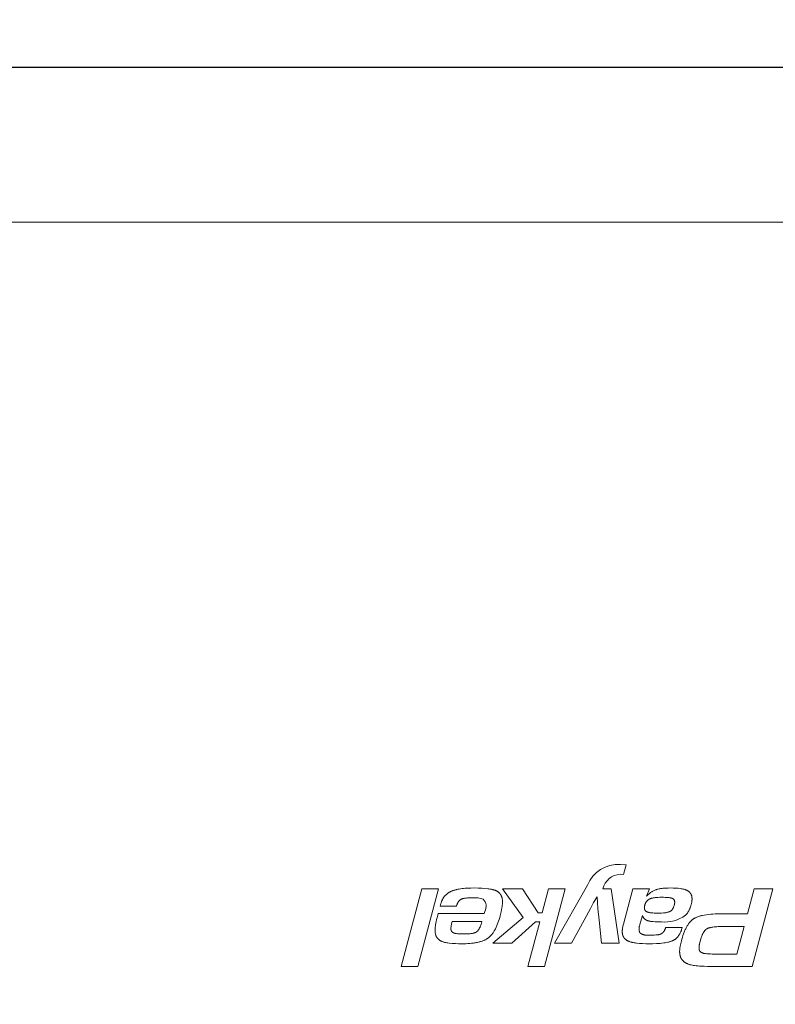
# Model space of a CAD drawing. Units: inches. Extents: x -1198 to -69, y -512 to 437.
# Tile 11 of 50: x -950.733 to -948.245, y 182.142 to 185.385. Entities that reach past the tile are written whole.
import ezdxf

# ---------------------------------------------------------------- set-up
doc = ezdxf.new("R2010")
doc.units = ezdxf.units.IN
doc.header["$MEASUREMENT"] = 0
for name, color, linetype, lineweight in [('0_Pen_No__7', 7, 'Continuous', 18), ('A-ANNO-DIMS', 2, 'Continuous', 18), ('A-EQPM', 60, 'Continuous', 18), ('A-FLOR-CASE', 7, 'Continuous', 25)]:
    doc.layers.add(name, color=color, linetype=linetype, lineweight=lineweight)
doc.styles.get("Standard").update_dxf_attribs({"font": 'arial.ttf'})
doc.dimstyles.get("Standard").update_dxf_attribs({"dimtxt": 6, "dimasz": 6, "dimexe": 0.18, "dimexo": 0.0625, "dimgap": 0.09, "dimtad": 0, "dimtih": 1, "dimtoh": 1, "dimdec": 0, "dimzin": 0, "dimdsep": 46, "dimlunit": 4, "dimtxsty": 'Standard', "dimblk": 'OBLIQUE', "dimcen": 0.09, "dimadec": 0, "dimazin": 0, "dimtfac": 1, "dimtdec": 0, "dimtofl": 0, "dimtmove": 0, "dimatfit": 3, "dimfxl": 1, "dimtolj": 1, "dimtzin": 0, "dimarcsym": 0})

# ---------------------------------------------------------------- blocks, each defined once
blk = doc.blocks.new('new block')
at = {"layer": '0_Pen_No__7'}
for p, q in [((-281.076, 68.7), (-279.346, 75.2)), ((-279.346, 75.2), (-275.605, 75.2)), ((-263.696, 68.7), (-261.965, 75.2)), ((-261.965, 75.2), (-260.589, 75.2)), ((-260.589, 75.2), (-261.574, 71.478)), ((-253.094, 68.7), (-251.364, 75.2)), ((-249.986, 75.2), (-251.716, 68.7)), ((-251.364, 75.2), (-249.986, 75.2)), ((-278.066, 74.168), (-278.675, 71.867)), ((-276.153, 74.168), (-278.066, 74.168)), ((-267.552, 68.7), (-268.209, 73.251)), ((-268.209, 73.251), (-266.747, 73.251)), ((-266.747, 73.251), (-266.552, 71.321)), ((-262.799, 73.251), (-265.577, 68.417)), ((-265.297, 71.321), (-264.224, 73.251)), ((-264.224, 73.251), (-262.799, 73.251)), ((-261.221, 71.478), (-259.224, 73.251)), ((-257.639, 73.251), (-260.186, 71.107)), ((-259.224, 73.251), (-257.639, 73.251)), ((-278.675, 71.867), (-276.921, 71.867)), ((-272.109, 71.935), (-273.497, 71.935)), ((-270.171, 70.951), (-269.953, 71.692)), ((-268.575, 71.673), (-269.367, 68.7)), ((-254.202, 71.634), (-254.141, 72.033)), ((-266.552, 71.321), (-266.443, 70.356)), ((-265.821, 70.356), (-265.297, 71.321)), ((-261.574, 71.478), (-261.221, 71.478)), ((-260.186, 71.107), (-258.444, 68.7)), ((-256.736, 71.458), (-254.251, 71.458)), ((-254.251, 71.458), (-254.202, 71.634)), ((-252.985, 71.146), (-253.081, 70.776)), ((-278.956, 70.795), (-279.517, 68.7)), ((-277.141, 70.795), (-278.956, 70.795)), ((-276.786, 70.805), (-277.141, 70.795)), ((-266.443, 70.356), (-266.393, 69.87)), ((-266.076, 69.87), (-265.821, 70.356)), ((-261.783, 70.717), (-262.318, 68.7)), ((-261.453, 70.717), (-261.783, 70.717)), ((-260.138, 68.7), (-261.453, 70.717)), ((-256.931, 70.776), (-256.98, 70.601)), ((-253.081, 70.776), (-256.931, 70.776)), ((-254.605, 70.152), (-253.239, 70.152)), ((-253.264, 70.065), (-253.277, 70.016)), ((-253.239, 70.152), (-253.264, 70.065)), ((-270.744, 68.7), (-270.512, 69.324)), ((-266.393, 69.87), (-266.37, 69.393)), ((-266.37, 69.393), (-266.076, 69.87)), ((-279.517, 68.7), (-281.076, 68.7)), ((-269.367, 68.7), (-270.744, 68.7)), ((-266.857, 68.7), (-267.552, 68.7)), ((-262.318, 68.7), (-263.696, 68.7)), ((-258.444, 68.7), (-260.138, 68.7)), ((-251.716, 68.7), (-253.094, 68.7)), ((-268.794, 66.703), (-268.575, 67.501)), ((-268.575, 67.501), (-268.307, 67.492)), ((-268.318, 66.683), (-268.794, 66.703))]:
    blk.add_line(p, q, dxfattribs=at)
blk.add_lwpolyline([(-354.492, 596.906), (481.176, 596.906, -0.414214), (485.681, 592.401), (485.681, 99.109), (486.244, 99.109), (486.244, 95.73), (485.681, 95.73), (485.681, 4.505, -0.414214), (481.176, 0), (-354.492, 0, -0.414214), (-358.997, 4.505), (-358.997, 95.73), (-359.56, 95.73), (-359.56, 99.109), (-358.997, 99.109), (-358.997, 592.401, -0.414214)], format="xyb", close=True, dxfattribs=at)
blk.add_lwpolyline([(-333.701, 12.952), (460.296, 12.952), (460.296, 570.439), (-333.701, 570.439)], close=True, dxfattribs=at)
for points in [[(-275.605, 75.2), (-275.335, 75.196), (-275.064, 75.185), (-274.929, 75.176), (-274.794, 75.164), (-274.659, 75.149), (-274.524, 75.132), (-274.432, 75.118), (-274.34, 75.102), (-274.249, 75.084), (-274.204, 75.074), (-274.159, 75.062), (-274.115, 75.05), (-274.071, 75.036), (-274.027, 75.022), (-273.983, 75.006), (-273.94, 74.989), (-273.898, 74.97), (-273.877, 74.96), (-273.856, 74.95), (-273.836, 74.939), (-273.815, 74.928), (-273.785, 74.911), (-273.755, 74.893), (-273.725, 74.874), (-273.696, 74.854), (-273.668, 74.833), (-273.64, 74.811), (-273.613, 74.789), (-273.586, 74.765), (-273.561, 74.741), (-273.537, 74.716), (-273.525, 74.703), (-273.513, 74.69), (-273.502, 74.677), (-273.49, 74.664), (-273.48, 74.65), (-273.469, 74.637), (-273.459, 74.623), (-273.449, 74.609), (-273.439, 74.594), (-273.43, 74.58), (-273.421, 74.565), (-273.412, 74.55), (-273.403, 74.534), (-273.394, 74.517), (-273.385, 74.5), (-273.377, 74.483), (-273.37, 74.466), (-273.362, 74.449), (-273.355, 74.431), (-273.349, 74.414), (-273.342, 74.396), (-273.336, 74.378), (-273.331, 74.36), (-273.326, 74.342), (-273.316, 74.305), (-273.307, 74.268), (-273.3, 74.23), (-273.294, 74.192), (-273.289, 74.154), (-273.285, 74.116), (-273.282, 74.077), (-273.279, 74.039), (-273.278, 74), (-273.277, 73.962), (-273.278, 73.905), (-273.28, 73.848), (-273.283, 73.792), (-273.288, 73.736), (-273.294, 73.68), (-273.302, 73.624), (-273.31, 73.569), (-273.32, 73.513), (-273.342, 73.403), (-273.367, 73.294), (-273.395, 73.185), (-273.425, 73.077)], [(-275.032, 72.969), (-274.96, 73.227), (-274.938, 73.314), (-274.929, 73.357), (-274.92, 73.401), (-274.913, 73.445), (-274.907, 73.489), (-274.902, 73.534), (-274.9, 73.556), (-274.899, 73.579), (-274.898, 73.602), (-274.898, 73.624), (-274.898, 73.647), (-274.898, 73.67), (-274.899, 73.687), (-274.9, 73.704), (-274.901, 73.722), (-274.903, 73.739), (-274.905, 73.756), (-274.908, 73.773), (-274.911, 73.789), (-274.915, 73.806), (-274.919, 73.822), (-274.923, 73.838), (-274.929, 73.854), (-274.935, 73.869), (-274.941, 73.884), (-274.949, 73.899), (-274.957, 73.913), (-274.966, 73.926), (-274.975, 73.938), (-274.984, 73.95), (-274.995, 73.961), (-275.006, 73.972), (-275.017, 73.982), (-275.029, 73.992), (-275.041, 74.002), (-275.054, 74.011), (-275.067, 74.02), (-275.081, 74.028), (-275.094, 74.036), (-275.108, 74.043), (-275.123, 74.05), (-275.137, 74.057), (-275.152, 74.064), (-275.166, 74.07), (-275.189, 74.078), (-275.212, 74.086), (-275.235, 74.094), (-275.258, 74.1), (-275.281, 74.106), (-275.305, 74.112), (-275.328, 74.116), (-275.352, 74.121), (-275.399, 74.128), (-275.446, 74.134), (-275.541, 74.143), (-275.694, 74.154), (-275.847, 74.162), (-276, 74.166), (-276.153, 74.168)], [(-276.921, 71.867), (-276.705, 71.869), (-276.488, 71.876), (-276.38, 71.882), (-276.272, 71.89), (-276.164, 71.901), (-276.056, 71.914), (-275.982, 71.925), (-275.908, 71.938), (-275.871, 71.946), (-275.834, 71.954), (-275.797, 71.963), (-275.761, 71.972), (-275.734, 71.98), (-275.708, 71.988), (-275.682, 71.997), (-275.656, 72.006), (-275.643, 72.011), (-275.63, 72.017), (-275.617, 72.022), (-275.605, 72.028), (-275.593, 72.034), (-275.58, 72.04), (-275.568, 72.047), (-275.556, 72.053), (-275.546, 72.06), (-275.535, 72.067), (-275.524, 72.074), (-275.514, 72.081), (-275.504, 72.089), (-275.494, 72.096), (-275.484, 72.104), (-275.474, 72.112), (-275.464, 72.121), (-275.455, 72.129), (-275.436, 72.146), (-275.418, 72.165), (-275.401, 72.183), (-275.381, 72.206), (-275.362, 72.229), (-275.343, 72.253), (-275.326, 72.277), (-275.309, 72.302), (-275.292, 72.327), (-275.277, 72.353), (-275.261, 72.379), (-275.242, 72.413), (-275.224, 72.449), (-275.206, 72.484), (-275.189, 72.52), (-275.173, 72.556), (-275.157, 72.593), (-275.128, 72.666), (-275.101, 72.741), (-275.077, 72.817), (-275.054, 72.893), (-275.032, 72.969)], [(-273.425, 73.077), (-273.465, 72.926), (-273.508, 72.776), (-273.555, 72.627), (-273.605, 72.479), (-273.66, 72.333), (-273.69, 72.261), (-273.72, 72.189), (-273.752, 72.118), (-273.786, 72.048), (-273.821, 71.978), (-273.857, 71.909), (-273.886, 71.856), (-273.916, 71.805), (-273.948, 71.753), (-273.98, 71.703), (-274.014, 71.653), (-274.049, 71.604), (-274.086, 71.557), (-274.124, 71.51), (-274.157, 71.471), (-274.192, 71.434), (-274.228, 71.397), (-274.264, 71.361), (-274.283, 71.344), (-274.303, 71.327), (-274.322, 71.311), (-274.342, 71.295), (-274.362, 71.279), (-274.382, 71.263), (-274.403, 71.249), (-274.424, 71.234), (-274.446, 71.219), (-274.469, 71.205), (-274.492, 71.191), (-274.515, 71.177), (-274.538, 71.164), (-274.562, 71.152), (-274.61, 71.128), (-274.659, 71.105), (-274.708, 71.084), (-274.759, 71.065), (-274.809, 71.046), (-274.873, 71.025), (-274.938, 71.004), (-275.002, 70.986), (-275.068, 70.969), (-275.133, 70.953), (-275.199, 70.938), (-275.331, 70.912), (-275.511, 70.882), (-275.692, 70.858), (-275.873, 70.84), (-276.056, 70.825), (-276.238, 70.816), (-276.421, 70.809), (-276.786, 70.805)], [(-273.497, 71.935), (-273.47, 72.026), (-273.441, 72.117), (-273.425, 72.162), (-273.409, 72.207), (-273.391, 72.252), (-273.373, 72.296), (-273.354, 72.339), (-273.334, 72.383), (-273.312, 72.425), (-273.29, 72.468), (-273.267, 72.509), (-273.243, 72.55), (-273.217, 72.59), (-273.191, 72.63), (-273.167, 72.662), (-273.143, 72.694), (-273.118, 72.726), (-273.092, 72.756), (-273.066, 72.786), (-273.038, 72.815), (-273.009, 72.842), (-272.995, 72.856), (-272.98, 72.869), (-272.951, 72.894), (-272.921, 72.917), (-272.891, 72.94), (-272.86, 72.961), (-272.829, 72.982), (-272.796, 73.001), (-272.764, 73.019), (-272.73, 73.037), (-272.71, 73.046), (-272.69, 73.056), (-272.65, 73.073), (-272.609, 73.09), (-272.567, 73.105), (-272.525, 73.119), (-272.483, 73.132), (-272.441, 73.145), (-272.398, 73.156), (-272.342, 73.17), (-272.287, 73.183), (-272.175, 73.206), (-272.063, 73.225), (-271.95, 73.242), (-271.796, 73.261), (-271.641, 73.276), (-271.485, 73.288), (-271.33, 73.297), (-271.019, 73.307), (-270.707, 73.31)], [(-270.854, 72.589), (-270.994, 72.587), (-271.133, 72.582), (-271.273, 72.573), (-271.413, 72.56), (-271.458, 72.554), (-271.503, 72.548), (-271.547, 72.541), (-271.569, 72.537), (-271.591, 72.532), (-271.612, 72.527), (-271.634, 72.521), (-271.655, 72.515), (-271.676, 72.508), (-271.686, 72.504), (-271.696, 72.5), (-271.706, 72.496), (-271.716, 72.491), (-271.726, 72.487), (-271.736, 72.482), (-271.746, 72.477), (-271.755, 72.472), (-271.77, 72.463), (-271.785, 72.454), (-271.8, 72.444), (-271.814, 72.434), (-271.828, 72.423), (-271.842, 72.411), (-271.855, 72.4), (-271.868, 72.388), (-271.881, 72.375), (-271.893, 72.362), (-271.905, 72.349), (-271.917, 72.336), (-271.928, 72.322), (-271.939, 72.308), (-271.949, 72.293), (-271.96, 72.279), (-271.973, 72.259), (-271.985, 72.239), (-271.997, 72.219), (-272.008, 72.198), (-272.019, 72.177), (-272.029, 72.156), (-272.039, 72.134), (-272.048, 72.113), (-272.057, 72.091), (-272.065, 72.069), (-272.081, 72.024), (-272.095, 71.98), (-272.109, 71.935)], [(-269.953, 71.692), (-269.937, 71.745), (-269.923, 71.797), (-269.91, 71.85), (-269.904, 71.876), (-269.899, 71.903), (-269.894, 71.93), (-269.89, 71.957), (-269.886, 71.984), (-269.883, 72.011), (-269.881, 72.038), (-269.879, 72.065), (-269.878, 72.093), (-269.878, 72.121), (-269.879, 72.136), (-269.879, 72.151), (-269.88, 72.166), (-269.881, 72.181), (-269.883, 72.196), (-269.885, 72.21), (-269.887, 72.225), (-269.89, 72.24), (-269.893, 72.254), (-269.897, 72.268), (-269.901, 72.282), (-269.906, 72.296), (-269.911, 72.309), (-269.917, 72.323), (-269.924, 72.335), (-269.931, 72.348), (-269.938, 72.359), (-269.946, 72.37), (-269.955, 72.381), (-269.964, 72.392), (-269.973, 72.402), (-269.983, 72.412), (-269.993, 72.421), (-270.004, 72.43), (-270.015, 72.439), (-270.026, 72.448), (-270.038, 72.456), (-270.05, 72.464), (-270.062, 72.471), (-270.074, 72.478), (-270.086, 72.485), (-270.098, 72.492), (-270.109, 72.498), (-270.12, 72.503), (-270.142, 72.513), (-270.164, 72.522), (-270.186, 72.531), (-270.209, 72.539), (-270.232, 72.546), (-270.255, 72.552), (-270.278, 72.558), (-270.301, 72.563), (-270.324, 72.568), (-270.348, 72.572), (-270.371, 72.576), (-270.395, 72.579), (-270.419, 72.581), (-270.467, 72.586), (-270.515, 72.588), (-270.564, 72.59), (-270.854, 72.589)], [(-270.707, 73.31), (-270.445, 73.307), (-270.183, 73.297), (-269.921, 73.28), (-269.659, 73.254), (-269.572, 73.243), (-269.484, 73.23), (-269.398, 73.215), (-269.354, 73.207), (-269.311, 73.198), (-269.268, 73.188), (-269.226, 73.176), (-269.184, 73.164), (-269.142, 73.151), (-269.1, 73.137), (-269.058, 73.121), (-269.017, 73.104), (-268.977, 73.085), (-268.949, 73.072), (-268.922, 73.058), (-268.895, 73.043), (-268.868, 73.027), (-268.842, 73.011), (-268.816, 72.994), (-268.791, 72.976), (-268.767, 72.957), (-268.743, 72.938), (-268.731, 72.928), (-268.72, 72.918), (-268.709, 72.907), (-268.698, 72.897), (-268.687, 72.886), (-268.677, 72.875), (-268.666, 72.864), (-268.656, 72.853), (-268.647, 72.841), (-268.637, 72.83), (-268.628, 72.818), (-268.619, 72.806), (-268.611, 72.793), (-268.602, 72.781), (-268.594, 72.768), (-268.586, 72.754), (-268.578, 72.741), (-268.571, 72.727), (-268.564, 72.713), (-268.557, 72.699), (-268.551, 72.685), (-268.545, 72.67), (-268.539, 72.655), (-268.534, 72.641), (-268.528, 72.626), (-268.523, 72.611), (-268.519, 72.596), (-268.514, 72.58), (-268.51, 72.565), (-268.506, 72.55), (-268.499, 72.518), (-268.494, 72.487), (-268.489, 72.455), (-268.484, 72.423), (-268.481, 72.391), (-268.479, 72.359), (-268.477, 72.327), (-268.477, 72.295), (-268.477, 72.255), (-268.478, 72.215), (-268.48, 72.175), (-268.483, 72.136), (-268.487, 72.097), (-268.492, 72.058), (-268.498, 72.019), (-268.504, 71.98), (-268.519, 71.902), (-268.536, 71.825), (-268.575, 71.673)], [(-258.26, 70.97), (-258.219, 71.12), (-258.175, 71.27), (-258.128, 71.418), (-258.077, 71.565), (-258.021, 71.711), (-257.992, 71.783), (-257.961, 71.854), (-257.929, 71.925), (-257.895, 71.995), (-257.86, 72.064), (-257.824, 72.133), (-257.794, 72.186), (-257.763, 72.239), (-257.732, 72.292), (-257.698, 72.343), (-257.664, 72.394), (-257.629, 72.444), (-257.592, 72.493), (-257.554, 72.54), (-257.519, 72.581), (-257.484, 72.62), (-257.448, 72.659), (-257.41, 72.696), (-257.371, 72.733), (-257.332, 72.767), (-257.311, 72.784), (-257.291, 72.801), (-257.27, 72.817), (-257.248, 72.833), (-257.226, 72.849), (-257.204, 72.864), (-257.181, 72.879), (-257.158, 72.894), (-257.111, 72.922), (-257.063, 72.948), (-257.014, 72.974), (-256.965, 72.997), (-256.914, 73.02), (-256.864, 73.041), (-256.803, 73.064), (-256.742, 73.086), (-256.681, 73.107), (-256.619, 73.126), (-256.557, 73.144), (-256.494, 73.16), (-256.368, 73.19), (-256.287, 73.207), (-256.205, 73.222), (-256.123, 73.236), (-256.04, 73.249), (-255.875, 73.27), (-255.709, 73.286), (-255.543, 73.297), (-255.376, 73.305), (-255.043, 73.31)], [(-255.226, 72.492), (-255.392, 72.49), (-255.475, 72.488), (-255.557, 72.484), (-255.64, 72.478), (-255.722, 72.47), (-255.804, 72.46), (-255.886, 72.448), (-255.944, 72.437), (-256.003, 72.424), (-256.032, 72.417), (-256.061, 72.41), (-256.089, 72.401), (-256.118, 72.392), (-256.14, 72.385), (-256.162, 72.377), (-256.184, 72.369), (-256.205, 72.36), (-256.215, 72.355), (-256.226, 72.35), (-256.236, 72.345), (-256.246, 72.339), (-256.256, 72.334), (-256.266, 72.328), (-256.276, 72.322), (-256.286, 72.315), (-256.294, 72.309), (-256.303, 72.303), (-256.312, 72.296), (-256.32, 72.29), (-256.328, 72.283), (-256.336, 72.275), (-256.344, 72.268), (-256.352, 72.261), (-256.36, 72.253), (-256.367, 72.245), (-256.382, 72.229), (-256.396, 72.213), (-256.41, 72.196), (-256.427, 72.175), (-256.443, 72.153), (-256.458, 72.13), (-256.473, 72.107), (-256.487, 72.084), (-256.501, 72.061), (-256.527, 72.013), (-256.544, 71.98), (-256.56, 71.947), (-256.576, 71.913), (-256.591, 71.879), (-256.619, 71.811), (-256.646, 71.741), (-256.67, 71.671), (-256.694, 71.6), (-256.736, 71.458)], [(-254.141, 72.033), (-254.141, 72.048), (-254.142, 72.063), (-254.143, 72.079), (-254.144, 72.094), (-254.146, 72.11), (-254.148, 72.125), (-254.151, 72.14), (-254.154, 72.155), (-254.157, 72.17), (-254.162, 72.185), (-254.166, 72.2), (-254.172, 72.214), (-254.178, 72.228), (-254.184, 72.242), (-254.191, 72.255), (-254.199, 72.268), (-254.207, 72.279), (-254.216, 72.29), (-254.224, 72.3), (-254.234, 72.31), (-254.244, 72.32), (-254.254, 72.329), (-254.264, 72.338), (-254.275, 72.347), (-254.287, 72.355), (-254.298, 72.363), (-254.31, 72.37), (-254.322, 72.377), (-254.335, 72.384), (-254.347, 72.391), (-254.36, 72.397), (-254.373, 72.403), (-254.382, 72.407), (-254.392, 72.411), (-254.411, 72.418), (-254.431, 72.425), (-254.451, 72.431), (-254.471, 72.436), (-254.491, 72.441), (-254.511, 72.445), (-254.531, 72.449), (-254.552, 72.453), (-254.572, 72.456), (-254.613, 72.461), (-254.696, 72.469), (-254.828, 72.479), (-254.961, 72.487), (-255.094, 72.491), (-255.226, 72.492)], [(-255.043, 73.31), (-254.777, 73.306), (-254.512, 73.296), (-254.246, 73.278), (-253.98, 73.251), (-253.892, 73.241), (-253.804, 73.229), (-253.716, 73.214), (-253.673, 73.205), (-253.63, 73.196), (-253.587, 73.186), (-253.545, 73.174), (-253.503, 73.161), (-253.461, 73.147), (-253.42, 73.132), (-253.4, 73.124), (-253.38, 73.115), (-253.36, 73.106), (-253.34, 73.097), (-253.32, 73.087), (-253.301, 73.077), (-253.273, 73.062), (-253.246, 73.045), (-253.219, 73.028), (-253.192, 73.01), (-253.167, 72.991), (-253.142, 72.972), (-253.117, 72.951), (-253.093, 72.93), (-253.07, 72.908), (-253.059, 72.897), (-253.048, 72.886), (-253.037, 72.874), (-253.027, 72.862), (-253.016, 72.85), (-253.006, 72.838), (-252.997, 72.826), (-252.987, 72.813), (-252.978, 72.801), (-252.969, 72.788), (-252.96, 72.775), (-252.951, 72.762), (-252.943, 72.748), (-252.935, 72.735), (-252.927, 72.719), (-252.918, 72.704), (-252.91, 72.688), (-252.903, 72.672), (-252.896, 72.655), (-252.889, 72.639), (-252.882, 72.622), (-252.876, 72.606), (-252.871, 72.589), (-252.865, 72.572), (-252.86, 72.555), (-252.855, 72.537), (-252.851, 72.52), (-252.846, 72.503), (-252.839, 72.467), (-252.832, 72.432), (-252.827, 72.396), (-252.822, 72.36), (-252.819, 72.324), (-252.816, 72.288), (-252.814, 72.251), (-252.813, 72.215), (-252.813, 72.179), (-252.814, 72.122), (-252.816, 72.065), (-252.82, 72.009), (-252.825, 71.953), (-252.832, 71.897), (-252.839, 71.842), (-252.856, 71.731), (-252.883, 71.584), (-252.914, 71.437), (-252.948, 71.291), (-252.985, 71.146)], [(-270.512, 69.324), (-270.556, 69.278), (-270.601, 69.234), (-270.646, 69.191), (-270.693, 69.149), (-270.741, 69.108), (-270.791, 69.069), (-270.841, 69.031), (-270.893, 68.995), (-270.941, 68.964), (-270.991, 68.934), (-271.041, 68.905), (-271.092, 68.878), (-271.144, 68.853), (-271.197, 68.83), (-271.251, 68.808), (-271.305, 68.788), (-271.335, 68.778), (-271.366, 68.768), (-271.429, 68.75), (-271.492, 68.734), (-271.555, 68.72), (-271.619, 68.708), (-271.684, 68.697), (-271.748, 68.688), (-271.813, 68.679), (-271.894, 68.67), (-271.975, 68.663), (-272.138, 68.652), (-272.324, 68.645), (-272.511, 68.642), (-272.735, 68.645), (-272.847, 68.649), (-272.958, 68.655), (-273.054, 68.662), (-273.149, 68.671), (-273.339, 68.693), (-273.411, 68.703), (-273.484, 68.715), (-273.556, 68.729), (-273.591, 68.736), (-273.627, 68.745), (-273.662, 68.754), (-273.697, 68.764), (-273.732, 68.775), (-273.766, 68.787), (-273.8, 68.8), (-273.834, 68.814), (-273.85, 68.822), (-273.867, 68.83), (-273.883, 68.838), (-273.9, 68.846), (-273.923, 68.859), (-273.946, 68.873), (-273.969, 68.887), (-273.991, 68.902), (-274.013, 68.918), (-274.034, 68.934), (-274.055, 68.951), (-274.075, 68.969), (-274.095, 68.987), (-274.104, 68.996), (-274.114, 69.006), (-274.123, 69.015), (-274.132, 69.025), (-274.141, 69.035), (-274.149, 69.045), (-274.158, 69.056), (-274.166, 69.066), (-274.174, 69.077), (-274.182, 69.087), (-274.189, 69.098), (-274.196, 69.109), (-274.203, 69.12), (-274.21, 69.132), (-274.217, 69.144), (-274.224, 69.156), (-274.23, 69.168), (-274.236, 69.18), (-274.242, 69.193), (-274.247, 69.205), (-274.253, 69.218), (-274.258, 69.231), (-274.262, 69.244), (-274.267, 69.257), (-274.271, 69.27), (-274.275, 69.283), (-274.283, 69.31), (-274.29, 69.337), (-274.295, 69.364), (-274.3, 69.392), (-274.304, 69.419), (-274.308, 69.447), (-274.31, 69.475), (-274.312, 69.503), (-274.313, 69.531), (-274.314, 69.558), (-274.313, 69.587), (-274.312, 69.615), (-274.311, 69.644), (-274.309, 69.672), (-274.306, 69.7), (-274.303, 69.728), (-274.295, 69.784), (-274.284, 69.848), (-274.272, 69.91), (-274.257, 69.973), (-274.241, 70.036), (-274.216, 70.124), (-274.188, 70.213), (-274.173, 70.256), (-274.157, 70.3), (-274.14, 70.343), (-274.123, 70.385), (-274.104, 70.428), (-274.084, 70.469), (-274.064, 70.511), (-274.042, 70.551), (-274.02, 70.592), (-273.996, 70.631), (-273.971, 70.67), (-273.946, 70.708), (-273.924, 70.737), (-273.902, 70.766), (-273.88, 70.795), (-273.856, 70.823), (-273.832, 70.85), (-273.808, 70.877), (-273.783, 70.903), (-273.757, 70.929)], [(-271.755, 71.478), (-271.579, 71.477), (-271.403, 71.472), (-271.227, 71.463), (-271.051, 71.451), (-270.936, 71.44), (-270.879, 71.433), (-270.822, 71.425), (-270.765, 71.415), (-270.737, 71.409), (-270.709, 71.403), (-270.681, 71.396), (-270.653, 71.388), (-270.625, 71.38), (-270.598, 71.371), (-270.579, 71.364), (-270.561, 71.357), (-270.542, 71.349), (-270.524, 71.342), (-270.506, 71.333), (-270.488, 71.325), (-270.47, 71.316), (-270.453, 71.306), (-270.436, 71.296), (-270.419, 71.285), (-270.403, 71.275), (-270.387, 71.263), (-270.371, 71.251), (-270.356, 71.239), (-270.341, 71.226), (-270.327, 71.212), (-270.313, 71.199), (-270.301, 71.185), (-270.288, 71.17), (-270.276, 71.155), (-270.265, 71.14), (-270.254, 71.124), (-270.243, 71.108), (-270.233, 71.091), (-270.223, 71.075), (-270.214, 71.058), (-270.206, 71.04), (-270.198, 71.023), (-270.19, 71.005), (-270.183, 70.987), (-270.177, 70.97), (-270.171, 70.951)], [(-253.277, 70.016), (-253.288, 69.973), (-253.301, 69.929), (-253.314, 69.886), (-253.328, 69.844), (-253.344, 69.801), (-253.36, 69.759), (-253.378, 69.717), (-253.396, 69.676), (-253.416, 69.635), (-253.436, 69.595), (-253.458, 69.555), (-253.481, 69.516), (-253.505, 69.478), (-253.53, 69.441), (-253.556, 69.404), (-253.583, 69.368), (-253.611, 69.335), (-253.639, 69.303), (-253.668, 69.271), (-253.698, 69.241), (-253.729, 69.211), (-253.76, 69.182), (-253.793, 69.154), (-253.826, 69.127), (-253.86, 69.101), (-253.895, 69.076), (-253.93, 69.052), (-253.966, 69.028), (-254.003, 69.006), (-254.04, 68.985), (-254.078, 68.964), (-254.116, 68.945), (-254.164, 68.922), (-254.212, 68.9), (-254.261, 68.88), (-254.311, 68.862), (-254.361, 68.844), (-254.412, 68.828), (-254.463, 68.813), (-254.514, 68.799), (-254.566, 68.786), (-254.618, 68.774), (-254.722, 68.753), (-254.827, 68.734), (-254.932, 68.718), (-255.069, 68.699), (-255.205, 68.684), (-255.341, 68.671), (-255.478, 68.661), (-255.637, 68.653), (-255.796, 68.647), (-256.115, 68.642), (-256.417, 68.645), (-256.568, 68.65), (-256.718, 68.658), (-256.971, 68.677), (-257.224, 68.703), (-257.317, 68.714), (-257.41, 68.728), (-257.502, 68.743), (-257.548, 68.752), (-257.593, 68.762), (-257.639, 68.773), (-257.684, 68.785), (-257.728, 68.798), (-257.772, 68.813), (-257.816, 68.829), (-257.837, 68.837), (-257.859, 68.846), (-257.88, 68.856), (-257.901, 68.866), (-257.922, 68.876), (-257.943, 68.887), (-257.972, 68.902), (-258.001, 68.919), (-258.029, 68.937), (-258.057, 68.955), (-258.084, 68.975), (-258.11, 68.995), (-258.136, 69.016), (-258.161, 69.038), (-258.173, 69.049), (-258.185, 69.061), (-258.197, 69.073), (-258.209, 69.084), (-258.22, 69.096), (-258.231, 69.109), (-258.242, 69.121), (-258.252, 69.134), (-258.263, 69.147), (-258.273, 69.16), (-258.282, 69.173), (-258.292, 69.186), (-258.301, 69.2), (-258.31, 69.214), (-258.318, 69.228), (-258.327, 69.242), (-258.335, 69.257), (-258.343, 69.272), (-258.351, 69.288), (-258.358, 69.304), (-258.365, 69.32), (-258.372, 69.336), (-258.378, 69.352), (-258.384, 69.369), (-258.39, 69.385), (-258.396, 69.402), (-258.406, 69.435), (-258.415, 69.469), (-258.423, 69.503), (-258.43, 69.542), (-258.437, 69.582), (-258.443, 69.621), (-258.447, 69.661), (-258.45, 69.701), (-258.453, 69.741), (-258.454, 69.781), (-258.455, 69.82), (-258.454, 69.882), (-258.451, 69.943), (-258.446, 70.004), (-258.441, 70.065), (-258.433, 70.126), (-258.425, 70.187), (-258.406, 70.309), (-258.375, 70.475), (-258.34, 70.641), (-258.26, 70.97)], [(-271.438, 70.747), (-271.611, 70.745), (-271.771, 70.739), (-271.917, 70.729), (-271.984, 70.723), (-272.048, 70.716), (-272.108, 70.708), (-272.164, 70.699), (-272.217, 70.688), (-272.267, 70.677), (-272.291, 70.671), (-272.314, 70.665), (-272.336, 70.658), (-272.358, 70.651), (-272.379, 70.644), (-272.399, 70.636), (-272.419, 70.629), (-272.438, 70.62), (-272.457, 70.612), (-272.474, 70.603), (-272.491, 70.593), (-272.508, 70.584), (-272.524, 70.574), (-272.54, 70.563), (-272.555, 70.552), (-272.57, 70.541), (-272.584, 70.529), (-272.598, 70.516), (-272.611, 70.503), (-272.624, 70.49), (-272.637, 70.476), (-272.649, 70.461), (-272.661, 70.446), (-272.672, 70.431), (-272.683, 70.414), (-272.694, 70.397), (-272.704, 70.38), (-272.715, 70.362), (-272.724, 70.343), (-272.734, 70.324), (-272.743, 70.305), (-272.752, 70.285), (-272.761, 70.265), (-272.769, 70.244), (-272.785, 70.202), (-272.8, 70.158), (-272.814, 70.114), (-272.824, 70.078), (-272.834, 70.042), (-272.842, 70.006), (-272.85, 69.97), (-272.853, 69.952), (-272.856, 69.934), (-272.859, 69.917), (-272.861, 69.899), (-272.862, 69.882), (-272.863, 69.865), (-272.864, 69.848), (-272.864, 69.832), (-272.864, 69.817), (-272.863, 69.802), (-272.862, 69.788), (-272.86, 69.773), (-272.858, 69.76), (-272.855, 69.746), (-272.852, 69.733), (-272.849, 69.72), (-272.845, 69.707), (-272.841, 69.694), (-272.836, 69.682), (-272.831, 69.67), (-272.825, 69.659), (-272.819, 69.648), (-272.813, 69.637), (-272.806, 69.626), (-272.799, 69.616), (-272.791, 69.606), (-272.783, 69.597), (-272.775, 69.587), (-272.766, 69.578), (-272.756, 69.57), (-272.746, 69.562), (-272.736, 69.554), (-272.725, 69.546), (-272.713, 69.538), (-272.701, 69.531), (-272.688, 69.525), (-272.675, 69.518), (-272.661, 69.512), (-272.647, 69.506), (-272.632, 69.5), (-272.617, 69.495), (-272.601, 69.49), (-272.584, 69.485), (-272.567, 69.481), (-272.549, 69.476), (-272.53, 69.472), (-272.491, 69.465), (-272.448, 69.458), (-272.403, 69.452), (-272.355, 69.446), (-272.304, 69.441), (-272.191, 69.433), (-272.067, 69.427), (-271.929, 69.423), (-271.78, 69.422)], [(-271.78, 69.422), (-271.607, 69.424), (-271.446, 69.431), (-271.3, 69.441), (-271.232, 69.448), (-271.168, 69.456), (-271.107, 69.465), (-271.049, 69.474), (-270.995, 69.485), (-270.969, 69.491), (-270.944, 69.497), (-270.92, 69.504), (-270.897, 69.511), (-270.874, 69.518), (-270.852, 69.525), (-270.83, 69.533), (-270.809, 69.541), (-270.789, 69.55), (-270.769, 69.558), (-270.749, 69.568), (-270.73, 69.578), (-270.711, 69.589), (-270.693, 69.6), (-270.676, 69.611), (-270.659, 69.623), (-270.642, 69.635), (-270.626, 69.648), (-270.61, 69.661), (-270.595, 69.675), (-270.581, 69.689), (-270.566, 69.704), (-270.552, 69.719), (-270.539, 69.734), (-270.526, 69.75), (-270.513, 69.767), (-270.5, 69.784), (-270.488, 69.802), (-270.476, 69.82), (-270.464, 69.838), (-270.453, 69.857), (-270.442, 69.877), (-270.432, 69.898), (-270.421, 69.919), (-270.411, 69.941), (-270.402, 69.963), (-270.393, 69.986), (-270.384, 70.009), (-270.376, 70.033), (-270.368, 70.056), (-270.354, 70.103), (-270.346, 70.132), (-270.339, 70.159), (-270.336, 70.173), (-270.334, 70.186), (-270.331, 70.198), (-270.33, 70.211), (-270.328, 70.227), (-270.328, 70.242), (-270.328, 70.256), (-270.328, 70.269), (-270.33, 70.305)], [(-270.33, 70.309), (-270.33, 70.324), (-270.331, 70.338), (-270.332, 70.353), (-270.333, 70.367), (-270.335, 70.381), (-270.337, 70.394), (-270.34, 70.408), (-270.343, 70.421), (-270.347, 70.433), (-270.351, 70.446), (-270.356, 70.458), (-270.361, 70.469), (-270.367, 70.481), (-270.373, 70.492), (-270.379, 70.503), (-270.386, 70.514), (-270.394, 70.524), (-270.402, 70.534), (-270.411, 70.544), (-270.42, 70.554), (-270.429, 70.563), (-270.439, 70.572), (-270.45, 70.581), (-270.461, 70.59), (-270.473, 70.598), (-270.486, 70.606), (-270.499, 70.614), (-270.512, 70.621), (-270.526, 70.629), (-270.541, 70.636), (-270.556, 70.643), (-270.572, 70.649), (-270.589, 70.656), (-270.606, 70.662), (-270.624, 70.668), (-270.642, 70.673), (-270.661, 70.679), (-270.681, 70.684), (-270.723, 70.694), (-270.767, 70.703), (-270.813, 70.711), (-270.863, 70.718), (-270.915, 70.724), (-270.97, 70.73), (-271.028, 70.735), (-271.152, 70.742), (-271.289, 70.746), (-271.438, 70.747)], [(-255.982, 69.46), (-255.827, 69.462), (-255.672, 69.467), (-255.518, 69.476), (-255.44, 69.483), (-255.362, 69.492), (-255.315, 69.498), (-255.267, 69.505), (-255.22, 69.513), (-255.196, 69.518), (-255.173, 69.523), (-255.149, 69.529), (-255.126, 69.535), (-255.104, 69.542), (-255.081, 69.55), (-255.059, 69.558), (-255.037, 69.567), (-255.026, 69.572), (-255.015, 69.577), (-255.005, 69.582), (-254.994, 69.587), (-254.978, 69.596), (-254.962, 69.605), (-254.947, 69.615), (-254.931, 69.625), (-254.916, 69.636), (-254.902, 69.647), (-254.888, 69.658), (-254.874, 69.67), (-254.866, 69.677), (-254.859, 69.684), (-254.845, 69.698), (-254.831, 69.713), (-254.818, 69.728), (-254.805, 69.744), (-254.792, 69.759), (-254.78, 69.776), (-254.769, 69.792), (-254.755, 69.813), (-254.742, 69.834), (-254.729, 69.855), (-254.717, 69.877), (-254.705, 69.899), (-254.694, 69.921), (-254.683, 69.943), (-254.673, 69.966), (-254.663, 69.989), (-254.654, 70.012), (-254.636, 70.058), (-254.62, 70.105), (-254.605, 70.152)]]:
    blk.add_lwpolyline(points, dxfattribs=at)
for centre, radius, start, end in [((-272.026, 68.543), 2.947, 84.73509, 125.96945), ((-256.236, 70.185), 0.852, 150.77527, 225.45817), ((-256.103, 71.739), 2.282, 251.32192, 273.04529), ((-268.106, 69.382), 2.707, 265.51181, 339.11597), ((-268.413, 69.092), 1.604, 273.78097, 345.86999)]:
    blk.add_arc(centre, radius, start, end, dxfattribs=at)
blk = doc.blocks.new('COUNTER-L')
at = {"ltscale": 10}
blk.add_line((49.3491, 23.9997), (0.0001, 23.9997), dxfattribs=at)
blk = doc.blocks.new('_Oblique')
at = {"color": 0, "linetype": 'ByBlock', "lineweight": -2}
blk.add_line((-0.5, -0.5), (0.5, 0.5), dxfattribs=at)
blk = doc.blocks.new('*D50')
at = {"layer": 'A-ANNO-DIMS', "color": 0, "lineweight": -2, "ltscale": 10, "transparency": 16777216}
for p, q in [((-978.4621, 185.2902), (-978.4621, 190.4026)), ((-945.1627, 185.2902), (-945.1627, 190.4026)), ((-978.4621, 190.2226), (-984.4621, 190.2226)), ((-945.1627, 190.2226), (-978.4621, 190.2226))]:
    blk.add_line(p, q, dxfattribs=at)
at = {"layer": 'DEFPOINTS', "color": 0, "ltscale": 10, "transparency": 16777216}
for p in [(-978.4621, 190.2226), (-978.4621, 185.2277), (-945.1627, 185.2277)]:
    blk.add_point(p, dxfattribs=at)
at = {"layer": 'A-ANNO-DIMS', "color": 0, "lineweight": -2, "ltscale": 10, "transparency": 16777216, "xscale": 6, "yscale": 6, "zscale": 6, "rotation": 180}
blk.add_blockref('_Oblique', (-978.4621, 190.2226), dxfattribs=at)
at = {"layer": 'A-ANNO-DIMS', "color": 0, "lineweight": -2, "ltscale": 10, "transparency": 16777216, "xscale": 6, "yscale": 6, "zscale": 6}
blk.add_blockref('_Oblique', (-945.1627, 190.2226), dxfattribs=at)
at = {"layer": 'A-ANNO-DIMS', "color": 0, "ltscale": 10, "transparency": 16777216, "insert": (-1009.2397, 190.2226), "char_height": 6, "attachment_point": 5}
blk.add_mtext('\\A1;HOB 33 TYP.', dxfattribs=at)

msp = doc.modelspace()

# ---------------------------------------------------------------- block references
at = {"layer": 'A-EQPM', "xscale": 0.0393700787401575, "yscale": 0.0393700787401575, "zscale": 0.0393700787401575, "rotation": 180}
msp.add_blockref('new block', (-959.3186, 185.2277), dxfattribs=at)
at = {"layer": 'A-FLOR-CASE'}
msp.add_blockref('COUNTER-L', (-988.751, 161.228), dxfattribs=at)

# ---------------------------------------------------------------- dimensions: what is measured, and where the dimension line sits
at = {"layer": 'A-ANNO-DIMS', "ltscale": 10}
dim = msp.add_linear_dim(base=(-978.4621, 190.2226), p1=(-945.1627, 185.2277), p2=(-978.4621, 185.2277), angle=180, text='HOB <> TYP.', dimstyle='Standard', override={"dimdec": 0, "dimlfac": 1, "dimrnd": 0, "dimzin": 0, "dimdsep": 46, "dimlunit": 2}, dxfattribs=at)
dim.commit()
dim.dimension.update_dxf_attribs({"geometry": '*D50', "text_midpoint": (-1009.2397, 190.2226)})

doc.saveas('drawing.dxf')
